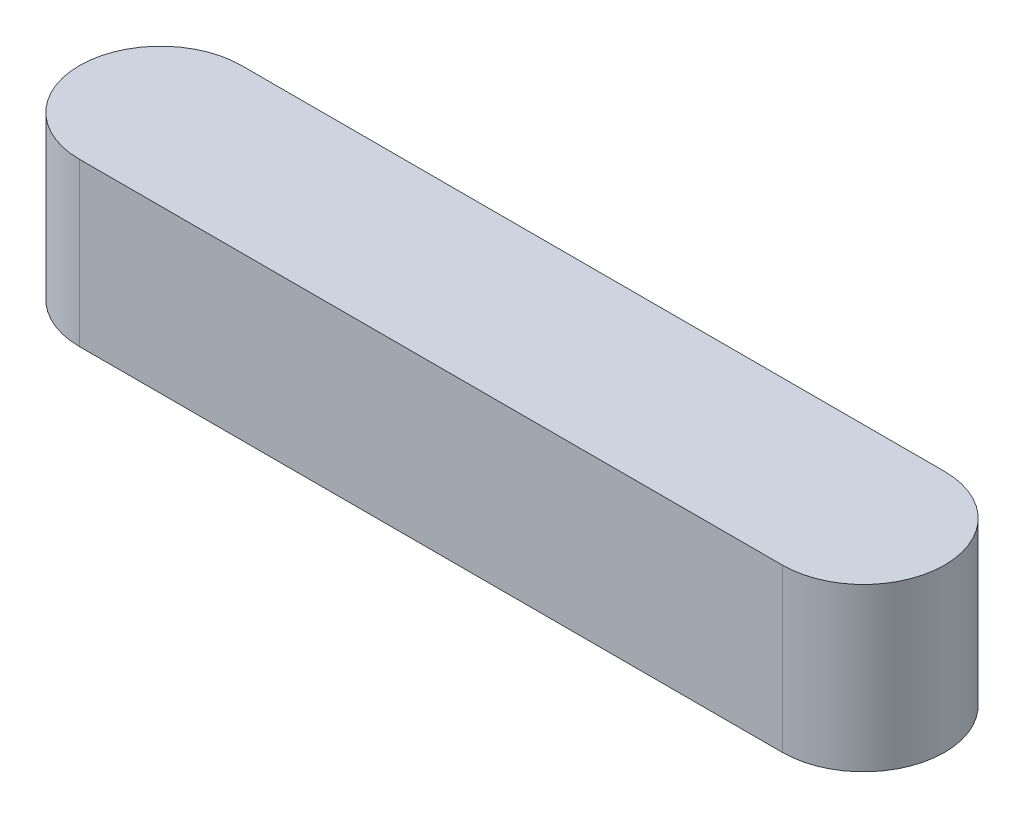
from build123d import *

# Parameters (mm, degrees)
KEY_BODY_6X6X32_DEPTH = 6


with BuildPart() as part:
    # Key Profile Slot 6x32 → Key Body 6x6x32 (new body)
    with BuildSketch(Plane(origin=(0, 0, 0), x_dir=(1, 0, 0), z_dir=(0, 1, 0))):
        with BuildLine():
            Line((-13, 3), (13, 3))
            ThreePointArc((13, 3), (16, 0), (13, -3))
            Line((13, -3), (-13, -3))
            ThreePointArc((-13, -3), (-16, 0), (-13, 3))
        make_face()
    extrude(amount=KEY_BODY_6X6X32_DEPTH)


solid = part.part
